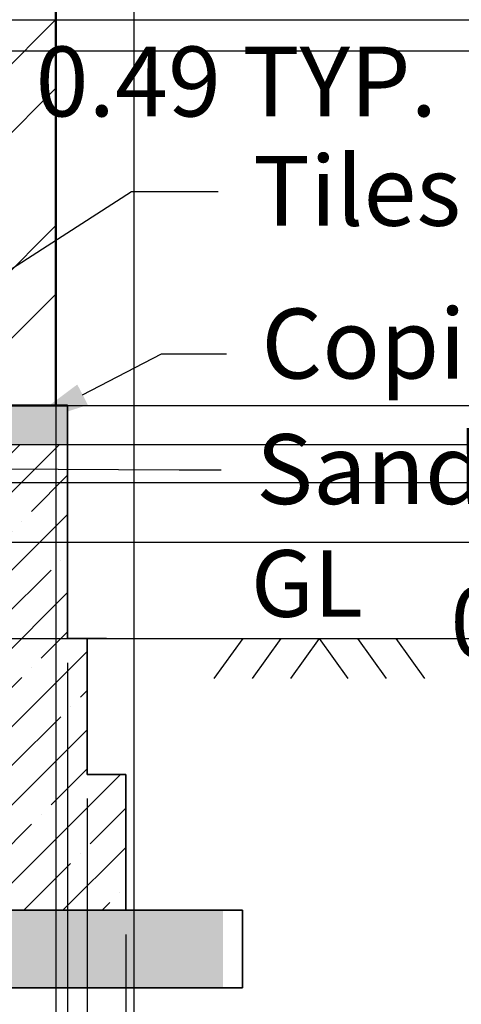
# Model space of a CAD drawing. Units: metres. Extents: x 22.1 to 34.4, y 4.4 to 12.4.
# Tile 6 of 8: x 31.7 to 32.8, y 7 to 9.5. Entities that reach past the tile are written whole.
import ezdxf
from ezdxf import colors
from ezdxf.entities.mleader import LeaderData, LeaderLine
from ezdxf.math import Vec2, Vec3

# ---------------------------------------------------------------- set-up
doc = ezdxf.new("R2010")
doc.units = ezdxf.units.M
doc.header["$MEASUREMENT"] = 0
for name, color, linetype, lineweight in [('A-ANNO-DIMS', 2, 'Continuous', 18), ('A-ANNO-TEXT', 7, 'Continuous', 18), ('A-FLOR', 3, 'Continuous', 25), ('A-WALL', 7, 'Continuous', 50), ('A-WALL-PATT', 8, 'Continuous', 18), ('C-TOPO', 3, 'Continuous', 25), ('S-FNDN', 1, 'Continuous', 35), ('S-FNDN-PATT', 8, 'Continuous', 13), ('S-SLAB-PATT', 8, 'Continuous', 13)]:
    doc.layers.add(name, color=color, linetype=linetype, lineweight=lineweight)
doc.styles.get("Standard").update_dxf_attribs({"font": 'arial.ttf'})
doc.dimstyles.get("Standard").update_dxf_attribs({"dimtxt": 0.18, "dimasz": 0.18, "dimexe": 0.18, "dimexo": 0.0625, "dimgap": 0.09, "dimtad": 0, "dimtih": 1, "dimtoh": 1, "dimzin": 0, "dimdsep": 46, "dimtxsty": 'Standard', "dimcen": 0.09, "dimadec": 0, "dimazin": 0, "dimtfac": 1, "dimtofl": 0, "dimtmove": 0, "dimatfit": 3, "dimfxl": 1, "dimtolj": 1, "dimtzin": 0, "dimarcsym": 0})

# ---------------------------------------------------------------- blocks, each defined once
blk = doc.blocks.new('*D7')
at = {"layer": 'A-ANNO-DIMS', "color": 0, "lineweight": -2, "transparency": 16777216}
for p, q in [((31.0581, 6.9474), (31.0581, 5.2806)), ((32.2581, 6.9474), (32.2581, 5.2806)), ((31.0581, 5.4606), (30.8781, 5.4606)), ((32.0781, 5.4606), (31.2381, 5.4606))]:
    blk.add_line(p, q, dxfattribs=at)
at = {"layer": 'A-ANNO-DIMS', "color": 0, "transparency": 16777216}
for points in [[(31.2381, 5.4906), (31.2381, 5.4306), (31.0581, 5.4606)], [(32.0781, 5.4906), (32.0781, 5.4306), (32.2581, 5.4606)]]:
    blk.add_solid(points, dxfattribs=at)
at = {"layer": 'Defpoints', "color": 0, "transparency": 16777216}
for p in [(31.0581, 7.0099), (32.2581, 7.0099), (32.2581, 5.4606)]:
    blk.add_point(p, dxfattribs=at)
at = {"layer": 'A-ANNO-DIMS', "color": 0, "transparency": 16777216, "insert": (30.5631, 5.4606), "char_height": 0.18, "attachment_point": 5}
blk.add_mtext('\\A1;1.20', dxfattribs=at)
blk = doc.blocks.new('*D8')
at = {"layer": 'A-ANNO-DIMS', "color": 0, "lineweight": -2, "transparency": 16777216}
for p, q in [((31.3581, 7.1474), (31.3581, 5.6208)), ((31.9581, 7.1474), (31.9581, 5.6208)), ((31.3581, 5.8008), (30.8904, 5.8008)), ((31.7781, 5.8008), (31.5381, 5.8008))]:
    blk.add_line(p, q, dxfattribs=at)
at = {"layer": 'A-ANNO-DIMS', "color": 0, "transparency": 16777216}
for points in [[(31.5381, 5.8308), (31.5381, 5.7708), (31.3581, 5.8008)], [(31.7781, 5.8308), (31.7781, 5.7708), (31.9581, 5.8008)]]:
    blk.add_solid(points, dxfattribs=at)
at = {"layer": 'Defpoints', "color": 0, "transparency": 16777216}
for p in [(31.3581, 7.2099), (31.9581, 7.2099), (31.9581, 5.8008)]:
    blk.add_point(p, dxfattribs=at)
at = {"layer": 'A-ANNO-DIMS', "color": 0, "transparency": 16777216, "insert": (30.5669, 5.8008), "char_height": 0.18, "attachment_point": 5}
blk.add_mtext('\\A1;0.60', dxfattribs=at)
blk = doc.blocks.new('*D9')
at = {"layer": 'A-ANNO-DIMS', "color": 0, "lineweight": -2, "transparency": 16777216}
for p, q in [((31.4581, 7.4974), (31.4581, 5.952)), ((31.8581, 7.4974), (31.8581, 5.952)), ((31.2781, 6.132), (30.8756, 6.132)), ((32.0381, 6.132), (32.2181, 6.132))]:
    blk.add_line(p, q, dxfattribs=at)
at = {"layer": 'A-ANNO-DIMS', "color": 0, "transparency": 16777216}
for points in [[(31.2781, 6.162), (31.2781, 6.102), (31.4581, 6.132)], [(32.0381, 6.162), (32.0381, 6.102), (31.8581, 6.132)]]:
    blk.add_solid(points, dxfattribs=at)
at = {"layer": 'Defpoints', "color": 0, "transparency": 16777216}
for p in [(31.4581, 7.5599), (31.8581, 7.5599), (31.8581, 6.132)]:
    blk.add_point(p, dxfattribs=at)
at = {"layer": 'A-ANNO-DIMS', "color": 0, "transparency": 16777216, "insert": (30.5521, 6.132), "char_height": 0.18, "attachment_point": 5}
blk.add_mtext('\\A1;0.40', dxfattribs=at)
blk = doc.blocks.new('*D10')
at = {"layer": 'A-ANNO-DIMS', "color": 0, "lineweight": -2, "transparency": 16777216}
for p, q in [((31.5081, 7.8474), (31.5081, 6.2035)), ((31.8081, 7.8474), (31.8081, 6.2035)), ((31.3281, 6.3835), (30.8854, 6.3835)), ((31.9881, 6.3835), (32.1681, 6.3835))]:
    blk.add_line(p, q, dxfattribs=at)
at = {"layer": 'A-ANNO-DIMS', "color": 0, "transparency": 16777216}
for points in [[(31.3281, 6.4135), (31.3281, 6.3535), (31.5081, 6.3835)], [(31.9881, 6.4135), (31.9881, 6.3535), (31.8081, 6.3835)]]:
    blk.add_solid(points, dxfattribs=at)
at = {"layer": 'Defpoints', "color": 0, "transparency": 16777216}
for p in [(31.5081, 7.9099), (31.8081, 7.9099), (31.8081, 6.3835)]:
    blk.add_point(p, dxfattribs=at)
at = {"layer": 'A-ANNO-DIMS', "color": 0, "transparency": 16777216, "insert": (30.562, 6.3835), "char_height": 0.18, "attachment_point": 5}
blk.add_mtext('\\A1;0.30', dxfattribs=at)
blk = doc.blocks.new('GROUND-SYMBOL')
for p, q in [((32.2587, 7.9099), (32.1846, 7.8067)), ((32.3571, 7.9099), (32.2831, 7.8067)), ((32.4556, 7.9099), (32.3816, 7.8067)), ((32.4556, 7.9099), (32.5296, 7.8067)), ((32.5541, 7.9099), (32.6281, 7.8067)), ((32.6525, 7.9099), (32.7266, 7.8067))]:
    blk.add_line(p, q)
blk = doc.blocks.new('*D18')
at = {"layer": 'A-ANNO-DIMS', "color": 0, "lineweight": -2, "transparency": 16777216}
for p, q in [((31.3118, 10.5649), (31.5885, 10.5649)), ((31.4085, 10.3849), (31.4085, 10.2175)), ((31.4085, 9.6839), (31.4085, 9.8513)), ((31.3118, 9.5039), (31.5885, 9.5039))]:
    blk.add_line(p, q, dxfattribs=at)
at = {"layer": 'A-ANNO-DIMS', "color": 0, "transparency": 16777216}
for points in [[(31.3785, 10.3849), (31.4385, 10.3849), (31.4085, 10.5649)], [(31.3785, 9.6839), (31.4385, 9.6839), (31.4085, 9.5039)]]:
    blk.add_solid(points, dxfattribs=at)
at = {"layer": 'Defpoints', "color": 0, "transparency": 16777216}
for p in [(31.2493, 10.5649), (31.4085, 10.5649), (31.2493, 9.5039)]:
    blk.add_point(p, dxfattribs=at)
at = {"layer": 'A-ANNO-DIMS', "color": 0, "transparency": 16777216, "insert": (31.4085, 10.0344), "char_height": 0.18, "attachment_point": 5}
blk.add_mtext('\\A1;WINDOW PANE 490 1.06 TYP.', dxfattribs=at)
blk = doc.blocks.new('*D19')
at = {"layer": 'A-ANNO-DIMS', "color": 0, "lineweight": -2, "transparency": 16777216}
for p, q in [((30.7603, 9.4414), (30.7603, 9.1648)), ((31.2493, 9.4414), (31.2493, 9.1648)), ((30.5803, 9.3448), (30.4003, 9.3448)), ((31.4293, 9.3448), (31.6093, 9.3448))]:
    blk.add_line(p, q, dxfattribs=at)
at = {"layer": 'A-ANNO-DIMS', "color": 0, "transparency": 16777216}
for points in [[(30.5803, 9.3748), (30.5803, 9.3148), (30.7603, 9.3448)], [(31.4293, 9.3748), (31.4293, 9.3148), (31.2493, 9.3448)]]:
    blk.add_solid(points, dxfattribs=at)
at = {"layer": 'Defpoints', "color": 0, "transparency": 16777216}
for p in [(30.7603, 9.5039), (31.2493, 9.5039), (31.2493, 9.3448)]:
    blk.add_point(p, dxfattribs=at)
at = {"layer": 'A-ANNO-DIMS', "color": 0, "transparency": 16777216, "insert": (32.2423, 9.3448), "char_height": 0.18, "attachment_point": 5}
blk.add_mtext('\\A1;0.49 TYP.', dxfattribs=at)
blk = doc.blocks.new('*D27')
at = {"layer": 'A-ANNO-DIMS', "color": 0, "lineweight": -2, "transparency": 16777216}
for p, q in [((31.5381, 11.4474), (31.5381, 6.2449)), ((31.7781, 11.4474), (31.7781, 6.2449)), ((31.3581, 6.4249), (31.1781, 6.4249)), ((31.9581, 6.4249), (32.1381, 6.4249))]:
    blk.add_line(p, q, dxfattribs=at)
at = {"layer": 'A-ANNO-DIMS', "color": 0, "transparency": 16777216}
for points in [[(31.3581, 6.4549), (31.3581, 6.3949), (31.5381, 6.4249)], [(31.9581, 6.4549), (31.9581, 6.3949), (31.7781, 6.4249)]]:
    blk.add_solid(points, dxfattribs=at)
at = {"layer": 'Defpoints', "color": 0, "transparency": 16777216}
for p in [(31.5381, 11.5099), (31.7781, 11.5099), (31.7781, 6.4249)]:
    blk.add_point(p, dxfattribs=at)
at = {"layer": 'A-ANNO-DIMS', "color": 0, "transparency": 16777216, "insert": (32.4615, 6.4249), "char_height": 0.18, "attachment_point": 5}
blk.add_mtext('\\A1;0.24', dxfattribs=at)
blk = doc.blocks.new('*D28')
at = {"layer": 'A-ANNO-DIMS', "color": 0, "lineweight": -2, "transparency": 16777216}
for p, q in [((31.7781, 11.4474), (31.7781, 6.2449)), ((31.9781, 11.4474), (31.9781, 6.2449)), ((31.5981, 6.4249), (31.4181, 6.4249)), ((32.1581, 6.4249), (32.3381, 6.4249))]:
    blk.add_line(p, q, dxfattribs=at)
at = {"layer": 'A-ANNO-DIMS', "color": 0, "transparency": 16777216}
for points in [[(31.5981, 6.4549), (31.5981, 6.3949), (31.7781, 6.4249)], [(32.1581, 6.4549), (32.1581, 6.3949), (31.9781, 6.4249)]]:
    blk.add_solid(points, dxfattribs=at)
at = {"layer": 'Defpoints', "color": 0, "transparency": 16777216}
for p in [(31.7781, 11.5099), (31.9781, 11.5099), (31.9781, 6.4249)]:
    blk.add_point(p, dxfattribs=at)
at = {"layer": 'A-ANNO-DIMS', "color": 0, "transparency": 16777216, "insert": (32.6615, 6.4249), "char_height": 0.18, "attachment_point": 5}
blk.add_mtext('\\A1;0.20', dxfattribs=at)
blk = doc.blocks.new('*D33')
at = {"layer": 'A-ANNO-DIMS', "color": 0, "lineweight": -2, "transparency": 16777216}
for p, q in [((31.5381, 11.4474), (31.5381, 6.2449)), ((31.3293, 10.5774), (31.3293, 6.2449)), ((31.1493, 6.4249), (30.9693, 6.4249)), ((31.7181, 6.4249), (31.8981, 6.4249))]:
    blk.add_line(p, q, dxfattribs=at)
at = {"layer": 'A-ANNO-DIMS', "color": 0, "transparency": 16777216}
for points in [[(31.1493, 6.4549), (31.1493, 6.3949), (31.3293, 6.4249)], [(31.7181, 6.4549), (31.7181, 6.3949), (31.5381, 6.4249)]]:
    blk.add_solid(points, dxfattribs=at)
at = {"layer": 'Defpoints', "color": 0, "transparency": 16777216}
for p in [(31.5381, 11.5099), (31.3293, 10.6399), (31.5381, 6.4249)]:
    blk.add_point(p, dxfattribs=at)
at = {"layer": 'A-ANNO-DIMS', "color": 0, "transparency": 16777216, "insert": (32.2045, 6.4249), "char_height": 0.18, "attachment_point": 5}
blk.add_mtext('\\A1;0.21', dxfattribs=at)
blk = doc.blocks.new('*D39')
at = {"layer": 'A-ANNO-DIMS', "color": 0, "lineweight": -2, "transparency": 16777216}
for p, q in [((31.2493, 9.4414), (31.2493, 6.2449)), ((31.3293, 9.3614), (31.3293, 6.2449)), ((31.0693, 6.4249), (30.8893, 6.4249)), ((31.5093, 6.4249), (31.6893, 6.4249))]:
    blk.add_line(p, q, dxfattribs=at)
at = {"layer": 'A-ANNO-DIMS', "color": 0, "transparency": 16777216}
for points in [[(31.0693, 6.4549), (31.0693, 6.3949), (31.2493, 6.4249)], [(31.5093, 6.4549), (31.5093, 6.3949), (31.3293, 6.4249)]]:
    blk.add_solid(points, dxfattribs=at)
at = {"layer": 'Defpoints', "color": 0, "transparency": 16777216}
for p in [(31.2493, 9.5039), (31.3293, 9.4239), (31.3293, 6.4249)]:
    blk.add_point(p, dxfattribs=at)
at = {"layer": 'A-ANNO-DIMS', "color": 0, "transparency": 16777216, "insert": (32.0133, 6.4249), "char_height": 0.18, "attachment_point": 5}
blk.add_mtext('\\A1;0.08', dxfattribs=at)
blk = doc.blocks.new('*D40')
at = {"layer": 'A-ANNO-DIMS', "color": 0, "lineweight": -2, "transparency": 16777216}
for p, q in [((31.3918, 10.6399), (33.8537, 10.6399)), ((33.6737, 10.4599), (33.6737, 10.2138)), ((33.6737, 9.6039), (33.6737, 9.85)), ((31.3918, 9.4239), (33.8537, 9.4239))]:
    blk.add_line(p, q, dxfattribs=at)
at = {"layer": 'A-ANNO-DIMS', "color": 0, "transparency": 16777216}
for points in [[(33.6437, 10.4599), (33.7037, 10.4599), (33.6737, 10.6399)], [(33.6437, 9.6039), (33.7037, 9.6039), (33.6737, 9.4239)]]:
    blk.add_solid(points, dxfattribs=at)
at = {"layer": 'Defpoints', "color": 0, "transparency": 16777216}
for p in [(31.3293, 10.6399), (31.3293, 9.4239), (33.6737, 9.4239)]:
    blk.add_point(p, dxfattribs=at)
at = {"layer": 'A-ANNO-DIMS', "color": 0, "transparency": 16777216, "insert": (33.6737, 10.0319), "char_height": 0.18, "attachment_point": 5}
blk.add_mtext('\\A1;1.216', dxfattribs=at)
blk = doc.blocks.new('*D42')
at = {"layer": 'A-ANNO-DIMS', "color": 0, "lineweight": -2, "transparency": 16777216}
for p, q in [((33.6737, 9.6839), (33.6737, 9.8639)), ((33.6737, 9.8639), (33.8537, 9.8639)), ((31.3118, 9.5039), (33.8537, 9.5039)), ((31.3918, 9.4239), (33.8537, 9.4239)), ((33.6737, 9.2439), (33.6737, 9.0639))]:
    blk.add_line(p, q, dxfattribs=at)
at = {"layer": 'A-ANNO-DIMS', "color": 0, "transparency": 16777216}
for points in [[(33.6437, 9.6839), (33.7037, 9.6839), (33.6737, 9.5039)], [(33.6437, 9.2439), (33.7037, 9.2439), (33.6737, 9.4239)]]:
    blk.add_solid(points, dxfattribs=at)
at = {"layer": 'Defpoints', "color": 0, "transparency": 16777216}
for p in [(31.2493, 9.5039), (33.6737, 9.5039), (31.3293, 9.4239)]:
    blk.add_point(p, dxfattribs=at)
at = {"layer": 'A-ANNO-DIMS', "color": 0, "transparency": 16777216, "insert": (34.1776, 9.8639), "char_height": 0.18, "attachment_point": 5}
blk.add_mtext('\\A1;0.08', dxfattribs=at)
blk = doc.blocks.new('*D43')
at = {"layer": 'A-ANNO-DIMS', "color": 0, "lineweight": -2, "transparency": 16777216}
for p, q in [((31.3918, 9.4239), (33.8537, 9.4239)), ((33.6737, 9.2439), (33.6737, 9.1488)), ((33.6737, 8.6899), (33.6737, 8.785)), ((31.5706, 8.5099), (33.8537, 8.5099))]:
    blk.add_line(p, q, dxfattribs=at)
at = {"layer": 'A-ANNO-DIMS', "color": 0, "transparency": 16777216}
for points in [[(33.6437, 9.2439), (33.7037, 9.2439), (33.6737, 9.4239)], [(33.6437, 8.6899), (33.7037, 8.6899), (33.6737, 8.5099)]]:
    blk.add_solid(points, dxfattribs=at)
at = {"layer": 'Defpoints', "color": 0, "transparency": 16777216}
for p in [(31.3293, 9.4239), (31.5081, 8.5099), (33.6737, 8.5099)]:
    blk.add_point(p, dxfattribs=at)
at = {"layer": 'A-ANNO-DIMS', "color": 0, "transparency": 16777216, "insert": (33.6737, 8.9669), "char_height": 0.18, "attachment_point": 5}
blk.add_mtext('\\A1;0.914', dxfattribs=at)
blk = doc.blocks.new('*D44')
at = {"layer": 'A-ANNO-DIMS', "color": 0, "lineweight": -2, "transparency": 16777216}
for p, q in [((33.6737, 8.6899), (33.6737, 8.8699)), ((24.8474, 8.5099), (33.8537, 8.5099)), ((24.5474, 8.4099), (33.8537, 8.4099)), ((33.6737, 8.2299), (33.6737, 8.0499)), ((33.6737, 8.0499), (33.4937, 8.0499))]:
    blk.add_line(p, q, dxfattribs=at)
at = {"layer": 'A-ANNO-DIMS', "color": 0, "transparency": 16777216}
for points in [[(33.6437, 8.6899), (33.7037, 8.6899), (33.6737, 8.5099)], [(33.6437, 8.2299), (33.7037, 8.2299), (33.6737, 8.4099)]]:
    blk.add_solid(points, dxfattribs=at)
at = {"layer": 'Defpoints', "color": 0, "transparency": 16777216}
for p in [(24.7849, 8.5099), (24.4849, 8.4099), (33.6737, 8.4099)]:
    blk.add_point(p, dxfattribs=at)
at = {"layer": 'A-ANNO-DIMS', "color": 0, "transparency": 16777216, "insert": (33.1702, 8.0499), "char_height": 0.18, "attachment_point": 5}
blk.add_mtext('\\A1;0.10', dxfattribs=at)
blk = doc.blocks.new('*D45')
at = {"layer": 'A-ANNO-DIMS', "color": 0, "lineweight": -2, "transparency": 16777216}
for p, q in [((33.6737, 8.5899), (33.6737, 8.7699)), ((24.5474, 8.4099), (33.8537, 8.4099)), ((24.8474, 8.3119), (33.8537, 8.3119)), ((33.6737, 8.1319), (33.6737, 7.9519)), ((33.6737, 7.9519), (33.4937, 7.9519))]:
    blk.add_line(p, q, dxfattribs=at)
at = {"layer": 'A-ANNO-DIMS', "color": 0, "transparency": 16777216}
for points in [[(33.6437, 8.5899), (33.7037, 8.5899), (33.6737, 8.4099)], [(33.6437, 8.1319), (33.7037, 8.1319), (33.6737, 8.3119)]]:
    blk.add_solid(points, dxfattribs=at)
at = {"layer": 'Defpoints', "color": 0, "transparency": 16777216}
for p in [(24.4849, 8.4099), (24.7849, 8.3119), (33.6737, 8.3119)]:
    blk.add_point(p, dxfattribs=at)
at = {"layer": 'A-ANNO-DIMS', "color": 0, "transparency": 16777216, "insert": (33.0998, 7.9519), "char_height": 0.18, "attachment_point": 5}
blk.add_mtext('\\A1;0.098', dxfattribs=at)
blk = doc.blocks.new('*D46')
at = {"layer": 'A-ANNO-DIMS', "color": 0, "lineweight": -2, "transparency": 16777216}
for p, q in [((33.6737, 8.4919), (33.6737, 8.6719)), ((24.8474, 8.3119), (33.8537, 8.3119)), ((24.8474, 8.1578), (33.8537, 8.1578)), ((33.6737, 7.9778), (33.6737, 7.7978)), ((33.6737, 7.7978), (33.4937, 7.7978))]:
    blk.add_line(p, q, dxfattribs=at)
at = {"layer": 'A-ANNO-DIMS', "color": 0, "transparency": 16777216}
for points in [[(33.6437, 8.4919), (33.7037, 8.4919), (33.6737, 8.3119)], [(33.6437, 7.9778), (33.7037, 7.9778), (33.6737, 8.1578)]]:
    blk.add_solid(points, dxfattribs=at)
at = {"layer": 'Defpoints', "color": 0, "transparency": 16777216}
for p in [(24.7849, 8.3119), (24.7849, 8.1578), (33.6737, 8.1578)]:
    blk.add_point(p, dxfattribs=at)
at = {"layer": 'A-ANNO-DIMS', "color": 0, "transparency": 16777216, "insert": (33.1692, 7.7978), "char_height": 0.18, "attachment_point": 5}
blk.add_mtext('\\A1;0.15', dxfattribs=at)
blk = doc.blocks.new('*D47')
at = {"layer": 'A-ANNO-DIMS', "color": 0, "lineweight": -2, "transparency": 16777216}
for p, q in [((33.6737, 8.3378), (33.6737, 8.5178)), ((24.8474, 8.1578), (33.8537, 8.1578)), ((24.8474, 7.9099), (33.8537, 7.9099)), ((33.6737, 7.7299), (33.6737, 7.5499)), ((33.6737, 7.5499), (33.4937, 7.5499))]:
    blk.add_line(p, q, dxfattribs=at)
at = {"layer": 'A-ANNO-DIMS', "color": 0, "transparency": 16777216}
for points in [[(33.6437, 8.3378), (33.7037, 8.3378), (33.6737, 8.1578)], [(33.6437, 7.7299), (33.7037, 7.7299), (33.6737, 7.9099)]]:
    blk.add_solid(points, dxfattribs=at)
at = {"layer": 'Defpoints', "color": 0, "transparency": 16777216}
for p in [(24.7849, 8.1578), (24.7849, 7.9099), (33.6737, 7.9099)]:
    blk.add_point(p, dxfattribs=at)
at = {"layer": 'A-ANNO-DIMS', "color": 0, "transparency": 16777216, "insert": (33.1692, 7.5499), "char_height": 0.18, "attachment_point": 5}
blk.add_mtext('\\A1;0.25', dxfattribs=at)

msp = doc.modelspace()

# ---------------------------------------------------------------- hatches: boundary and pattern name
at = {"layer": 'A-WALL-PATT'}
h = msp.add_hatch(dxfattribs=at)
h.set_pattern_fill('ANSI32', color=256)
h.paths.add_polyline_path([(24.7549, 11.5099), (24.5149, 11.5099), (24.5149, 11.1399), (24.7549, 11.1399)])
h.paths.add_polyline_path([(24.7549, 10.6399), (24.5149, 10.6399), (24.5149, 8.5099), (24.6349, 8.5099), (24.7549, 8.5099)])
h.paths.add_polyline_path([(26.5706, 11.5099), (26.4206, 11.5099), (26.4206, 8.5099), (26.5706, 8.5099)])
h.paths.add_polyline_path([(28.0901, 10.6399), (28.0901, 11.5099), (27.8501, 11.5099), (27.8501, 8.5099), (28.0901, 8.5099)])
h.paths.add_polyline_path([(31.7781, 11.5099), (31.5381, 11.5099), (31.5381, 8.5099), (31.6581, 8.5099), (31.7781, 8.5099)])
at = {"layer": 'S-FNDN-PATT'}
h = msp.add_hatch(dxfattribs=at)
h.set_pattern_fill('ANSI35', color=256, scale=0.57)
h.paths.add_polyline_path([(24.3849, 7.5599), (24.2849, 7.5599), (24.2849, 7.2099), (24.9849, 7.2099), (24.9849, 7.5599), (24.8849, 7.5599), (24.8849, 7.9099), (24.7849, 7.9099), (24.7849, 8.4099), (24.4849, 8.4099), (24.4849, 7.9099), (24.3849, 7.9099)])
h.paths.add_polyline_path([(27.7201, 7.5599), (27.6201, 7.5599), (27.6201, 7.2099), (28.3201, 7.2099), (28.3201, 7.5599), (28.2201, 7.5599), (28.2201, 7.9099), (28.1201, 7.9099), (28.1201, 8.4099), (27.8201, 8.4099), (27.8201, 7.9099), (27.7201, 7.9099)])
h.paths.add_polyline_path([(26.7456, 7.9099), (26.6456, 7.9099), (26.6456, 8.4099), (26.3456, 8.4099), (26.3456, 7.9099), (26.2456, 7.9099), (26.2456, 7.5599), (26.4616, 7.5599), (26.4616, 7.6127), (26.4825, 7.5003), (26.4825, 7.5599), (26.7456, 7.5599)])
h.paths.add_polyline_path([(31.8581, 7.5599), (31.8581, 7.9099), (31.8081, 7.9099), (31.8081, 8.4099), (31.5081, 8.4099), (31.5081, 7.9099), (31.4581, 7.9099), (31.4581, 7.5599), (31.3581, 7.5599), (31.3581, 7.2099), (31.9581, 7.2099), (31.9581, 7.5599)])
at = {"layer": 'S-SLAB-PATT'}
h = msp.add_hatch(dxfattribs=at)
h.set_pattern_fill('AR-CONC', color=256, scale=0.04)
h.set_pattern_definition([(50, (0, 0), (0.286904, -0.0251009), [0.03, -0.33]), (355, (0, 0), (-0.0555005, 0.3008769), [0.024, -0.264]), (100.4514, (0.0239, -0.0021), (0.2314035, 0.275776), [0.025496, -0.2804568]), (46.1842, (0, 0.08), (0.4268965, -0.0662077), [0.045, -0.495]), (96.6356, (0.03557, 0.0745), (0.373865, 0.3896474), [0.038244, -0.4206855]), (351.1842, (0, 0.08), (0.373865, 0.3896474), [0.036, -0.396]), (21, (0.04, 0.06), (0.2387628, -0.1610476), [0.03, -0.33]), (326, (0.04, 0.06), (0.0973261, 0.29006), [0.024, -0.264]), (71.4514, (0.0599, 0.04658), (0.336089, 0.1290125), [0.025496, -0.2804568]), (37.5, (0, 0), (0.00486394, 0.13315754), [0, -0.2608, 0, -0.268, 0, -0.265]), (7.5, (0, 0), (0.1052278, 0.1577647), [0, -0.1528, 0, -0.2548, 0, -0.101]), (327.5, (-0.0892, 0), (0.21352897, -0.00902195), [0, -0.1, 0, -0.312, 0, -0.414]), (317.5, (-0.1292, 0), (0.2332745, 0.040042), [0, -0.13, 0, -0.2072, 0, -0.294])])
h.paths.add_polyline_path([(31.9781, 11.6599), (24.3149, 11.6599), (24.3149, 11.5099), (24.5149, 11.5099), (31.7781, 11.5099), (31.9781, 11.5099)])
h.paths.add_polyline_path([(25.1849, 7.2099), (24.9849, 7.2099), (24.0849, 7.2099), (24.0849, 7.0099), (25.1849, 7.0099)])
h.paths.add_polyline_path([(32.2081, 7.2099), (32.0081, 7.2099), (31.1081, 7.2099), (31.1081, 7.0099), (32.2081, 7.0099)])
h.paths.add_polyline_path([(28.5201, 7.2099), (28.3201, 7.2099), (27.4201, 7.2099), (27.4201, 7.0099), (28.5201, 7.0099)])
h.paths.add_polyline_path([(24.7849, 8.5099), (24.6349, 8.5099), (24.5149, 8.5099), (24.4849, 8.5099), (24.4849, 8.4099), (24.7849, 8.4099)])
h.paths.add_polyline_path([(26.6456, 8.5099), (26.3456, 8.5099), (26.3456, 8.4099), (26.6456, 8.4099)])
h.paths.add_polyline_path([(28.1201, 8.5099), (28.0901, 8.5099), (27.8201, 8.5099), (27.8201, 8.4099), (28.1201, 8.4099)])
h.paths.add_polyline_path([(31.8081, 8.5099), (31.6581, 8.5099), (31.5381, 8.5099), (31.5081, 8.5099), (31.5081, 8.4099), (31.8081, 8.4099)])
h.paths.add_polyline_path([(26.3456, 8.3119), (24.7849, 8.3119), (24.7849, 8.1578), (26.3456, 8.1578)])
h.paths.add_polyline_path([(27.8201, 8.3119), (26.6456, 8.3119), (26.6456, 8.1578), (27.8201, 8.1578)])
h.paths.add_polyline_path([(31.5081, 8.3119), (28.1201, 8.3119), (28.1201, 8.1578), (31.5081, 8.1578)])

# ---------------------------------------------------------------- linework, layer by layer
at = {"layer": 'A-FLOR'}
msp.add_line((28.1201, 8.4099), (31.8081, 8.4099), dxfattribs=at)
at = {"layer": 'A-WALL'}
for p, q in [((31.7781, 8.5099), (31.7781, 11.5099)), ((31.8081, 8.5099), (31.6581, 8.5099)), ((31.6581, 8.5099), (31.7781, 8.5099))]:
    msp.add_line(p, q, dxfattribs=at)
at = {"layer": 'C-TOPO'}
msp.add_line((31.9081, 7.9099), (33.0887, 7.9099), dxfattribs=at)
at = {"layer": 'S-FNDN'}
for p, q in [((31.8081, 7.9099), (31.8081, 8.5099)), ((31.9081, 7.9099), (31.8081, 7.9099)), ((31.8581, 7.5599), (31.8581, 7.9099)), ((31.9581, 7.5599), (31.8581, 7.5599)), ((31.9581, 7.2099), (31.9581, 7.5599)), ((31.0581, 7.2099), (32.0081, 7.2099)), ((32.2581, 7.2099), (32.0081, 7.2099)), ((32.2581, 7.0099), (32.2581, 7.2099)), ((31.0581, 7.0099), (32.2581, 7.0099))]:
    msp.add_line(p, q, dxfattribs=at)

# ---------------------------------------------------------------- block references
at = {"layer": 'C-TOPO'}
msp.add_blockref('GROUND-SYMBOL', (0, 0), dxfattribs=at)

# ---------------------------------------------------------------- texts
at = {"layer": 'A-ANNO-TEXT', "insert": (32.28, 8.1374), "char_height": 0.1716, "attachment_point": 1}
msp.add_mtext_dynamic_manual_height_columns('GL', width=0.269561, gutter_width=0.858, heights=[0], dxfattribs=at)

# ---------------------------------------------------------------- dimensions: what is measured, and where the dimension line sits
at = {"layer": 'A-ANNO-DIMS'}
for base, p1, p2, picture, middle in [((31.5381, 6.4249), (31.3293, 10.6399), (31.5381, 11.5099), '*D33', (32.2045, 6.4249)), ((31.7781, 6.4249), (31.5381, 11.5099), (31.7781, 11.5099), '*D27', (32.4615, 6.4249)), ((31.9781, 6.4249), (31.7781, 11.5099), (31.9781, 11.5099), '*D28', (32.6615, 6.4249)), ((31.3293, 6.4249), (31.2493, 9.5039), (31.3293, 9.4239), '*D39', (32.0133, 6.4249))]:
    dim = msp.add_linear_dim(base=base, p1=p1, p2=p2, dimstyle='Standard', override={"dimdec": 2, "dimlfac": 1, "dimrnd": 0, "dimzin": 0, "dimdsep": 46, "dimlunit": 2}, dxfattribs=at)
    dim.commit()
    dim.dimension.update_dxf_attribs({"geometry": picture, "text_midpoint": middle})
dim = msp.add_linear_dim(base=(31.4085, 10.5649), p1=(31.2493, 9.5039), p2=(31.2493, 10.5649), angle=90, text='WINDOW PANE 490 <> TYP.', dimstyle='Standard', override={"dimdec": 2, "dimrnd": 0, "dimzin": 0, "dimlunit": 2}, dxfattribs=at)
dim.commit()
dim.dimension.update_dxf_attribs({"geometry": '*D18', "text_midpoint": (31.4085, 10.0344)})
for base, p1, p2, override, picture, middle in [((33.6737, 9.4239), (31.3293, 10.6399), (31.3293, 9.4239), {"dimdec": 3, "dimlfac": 1, "dimrnd": 0, "dimzin": 0, "dimdsep": 46, "dimlunit": 2}, '*D40', (33.6737, 10.0319)), ((33.6737, 9.5039), (31.3293, 9.4239), (31.2493, 9.5039), {"dimdec": 2, "dimlfac": 1, "dimrnd": 0, "dimzin": 0, "dimdsep": 46, "dimlunit": 2}, '*D42', (34.1776, 9.8639)), ((33.6737, 8.5099), (31.3293, 9.4239), (31.5081, 8.5099), {"dimdec": 3, "dimlfac": 1, "dimrnd": 0, "dimzin": 0, "dimdsep": 46, "dimlunit": 2}, '*D43', (33.6737, 8.9669)), ((33.6737, 8.4099), (24.7849, 8.5099), (24.4849, 8.4099), {"dimdec": 2, "dimlfac": 1, "dimrnd": 0, "dimzin": 0, "dimdsep": 46, "dimlunit": 2}, '*D44', (33.1702, 8.0499)), ((33.6737, 8.3119), (24.4849, 8.4099), (24.7849, 8.3119), {"dimdec": 3, "dimlfac": 1, "dimrnd": 0, "dimzin": 0, "dimdsep": 46, "dimlunit": 2}, '*D45', (33.0998, 7.9519)), ((33.6737, 8.1578), (24.7849, 8.3119), (24.7849, 8.1578), {"dimdec": 2, "dimlfac": 1, "dimrnd": 0, "dimzin": 0, "dimdsep": 46, "dimlunit": 2}, '*D46', (33.1692, 7.7978)), ((33.6737, 7.9099), (24.7849, 8.1578), (24.7849, 7.9099), {"dimdec": 2, "dimlfac": 1, "dimrnd": 0, "dimzin": 0, "dimdsep": 46, "dimlunit": 2}, '*D47', (33.1692, 7.5499))]:
    dim = msp.add_linear_dim(base=base, p1=p1, p2=p2, angle=90, dimstyle='Standard', override=override, dxfattribs=at)
    dim.commit()
    dim.dimension.update_dxf_attribs({"geometry": picture, "text_midpoint": middle})
dim = msp.add_linear_dim(base=(31.2493, 9.3448), p1=(30.7603, 9.5039), p2=(31.2493, 9.5039), text='<> TYP.', dimstyle='Standard', override={"dimdec": 2, "dimrnd": 0, "dimzin": 0, "dimlunit": 2}, dxfattribs=at)
dim.commit()
dim.dimension.update_dxf_attribs({"geometry": '*D19', "text_midpoint": (32.2423, 9.3448)})
for base, p1, p2, picture, middle in [((31.8081, 6.3835), (31.5081, 7.9099), (31.8081, 7.9099), '*D10', (30.562, 6.3835)), ((31.8581, 6.132), (31.4581, 7.5599), (31.8581, 7.5599), '*D9', (30.5521, 6.132)), ((31.9581, 5.8008), (31.3581, 7.2099), (31.9581, 7.2099), '*D8', (30.5669, 5.8008)), ((32.2581, 5.4606), (31.0581, 7.0099), (32.2581, 7.0099), '*D7', (30.5631, 5.4606))]:
    dim = msp.add_linear_dim(base=base, p1=p1, p2=p2, dimstyle='Standard', override={"dimclrd": 0, "dimclre": 0, "dimclrt": 0}, dxfattribs=at)
    dim.commit()
    dim.dimension.update_dxf_attribs({"geometry": picture, "text_midpoint": middle, "dimtype": 160})

# ---------------------------------------------------------------- leaders
at = {"layer": 'A-ANNO-TEXT'}
ml = msp.add_multileader_mtext('Standard', dxfattribs=at)
ml.set_content('Tiles', color=256)
ml.set_leader_properties()
ml.build(insert=Vec2(0, 0))
ml.multileader.update_dxf_attribs({"dogleg_length": 0.36, "arrow_head_size": 0.18})
ctx = ml.context
ctx.base_point, ctx.char_height, ctx.arrow_head_size, ctx.landing_gap_size, ctx.plane_origin = Vec3(32.1951, 9.0617), 0.18, 0.18, 0.09, Vec3(31.1169, 8.5099)
notes = []
notes.append((ctx, [(0, (1, 1, 0), (31.9729, 9.0617), (1, 0), 0.2223, [(0, [(31.1169, 8.5099)], 0, [])])]))
ctx.mtext.insert, ctx.mtext.flow_direction = Vec3(32.2851, 9.1532), 5
ml = msp.add_multileader_mtext('Standard', dxfattribs=at)
ml.set_content('Coping', color=256)
ml.set_leader_properties()
ml.build(insert=Vec2(0, 0))
ml.multileader.update_dxf_attribs({"dogleg_length": 0.36, "arrow_head_size": 0.18})
ctx = ml.context
ctx.base_point, ctx.char_height, ctx.arrow_head_size, ctx.landing_gap_size, ctx.plane_origin = Vec3(32.2169, 8.6432), 0.18, 0.18, 0.09, Vec3(31.6868, 8.4551)
notes.append((ctx, [(0, (1, 1, 0), (32.0498, 8.6432), (1, 0), 0.1671, [(0, [(31.6868, 8.4551)], 0, [])])]))
ctx.mtext.insert, ctx.mtext.flow_direction = Vec3(32.3069, 8.7596), 5
ml = msp.add_multileader_mtext('Standard', dxfattribs=at)
ml.set_content('Sand bed', color=256)
ml.set_leader_properties()
ml.build(insert=Vec2(0, 0))
ml.multileader.update_dxf_attribs({"dogleg_length": 0.36, "arrow_head_size": 0.18})
ctx = ml.context
ctx.base_point, ctx.char_height, ctx.arrow_head_size, ctx.landing_gap_size, ctx.plane_origin = Vec3(32.2032, 8.3447), 0.18, 0.18, 0.09, Vec3(31.4464, 8.3479)
notes.append((ctx, [(0, (1, 1, 0), (32.0951, 8.3447), (1, 0), 0.1082, [(0, [(31.4464, 8.3479)], 0, [])])]))
ctx.mtext.insert, ctx.mtext.flow_direction = Vec3(32.2932, 8.4363), 5
for ctx, leaders in notes:
    for number, flags, end, landing, length, lines in leaders:
        leader = LeaderData()
        leader.index, (leader.has_last_leader_line, leader.has_dogleg_vector, leader.attachment_direction) = number, flags
        leader.last_leader_point, leader.dogleg_vector, leader.dogleg_length = Vec3(end), Vec3(landing), length
        for number, points, colour, breaks in lines:
            line = LeaderLine()
            line.index, line.vertices, line.color, line.breaks = number, Vec3.list(points), colors.encode_raw_color(colour), breaks
            leader.lines.append(line)
        ctx.leaders.append(leader)

doc.saveas('drawing.dxf')
